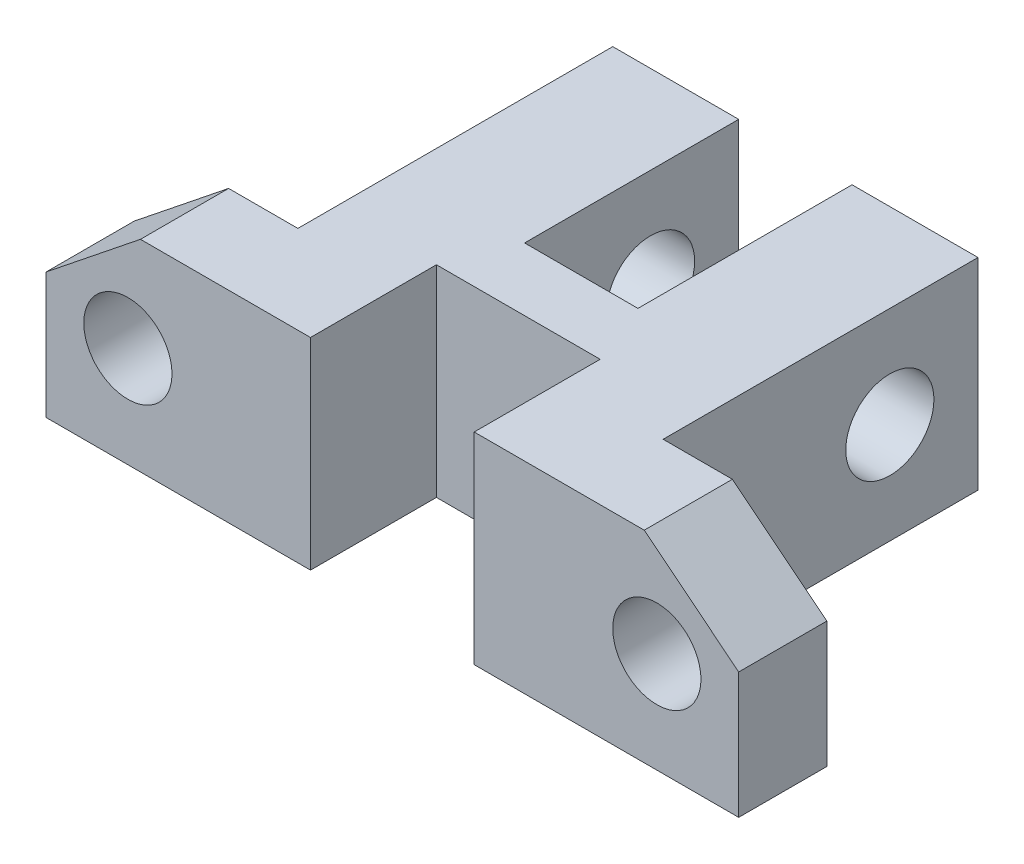
ISO-10303-21;
HEADER;
FILE_DESCRIPTION(('STEP AP214'),'2;1');
FILE_NAME('part.step','',(''),(''),'','','');
FILE_SCHEMA(('AUTOMOTIVE_DESIGN { 1 0 10303 214 1 1 1 1 }'));
ENDSEC;
DATA;
#1=APPLICATION_CONTEXT('core data for automotive mechanical design processes');
#2=APPLICATION_PROTOCOL_DEFINITION('international standard','automotive_design',2000,#1);
#3=PRODUCT_CONTEXT('',#1,'mechanical');
#4=PRODUCT('Part','Part','',(#3));
#5=PRODUCT_RELATED_PRODUCT_CATEGORY('part','',(#4));
#6=PRODUCT_DEFINITION_FORMATION('','',#4);
#7=PRODUCT_DEFINITION_CONTEXT('part definition',#1,'design');
#8=PRODUCT_DEFINITION('design','',#6,#7);
#9=PRODUCT_DEFINITION_SHAPE('','',#8);
#10=(LENGTH_UNIT() NAMED_UNIT(*) SI_UNIT(.MILLI.,.METRE.));
#11=(NAMED_UNIT(*) PLANE_ANGLE_UNIT() SI_UNIT($,.RADIAN.));
#12=(NAMED_UNIT(*) SI_UNIT($,.STERADIAN.) SOLID_ANGLE_UNIT());
#13=UNCERTAINTY_MEASURE_WITH_UNIT(LENGTH_MEASURE(1.E-05),#10,'distance_accuracy_value','');
#14=(GEOMETRIC_REPRESENTATION_CONTEXT(3) GLOBAL_UNCERTAINTY_ASSIGNED_CONTEXT((#13)) GLOBAL_UNIT_ASSIGNED_CONTEXT((#10,
#11,#12)) REPRESENTATION_CONTEXT('',''));
#15=CARTESIAN_POINT('',(0.,0.,0.));
#16=DIRECTION('',(0.,0.,1.));
#17=DIRECTION('',(1.,0.,0.));
#18=AXIS2_PLACEMENT_3D('',#15,#16,#17);
#19=CARTESIAN_POINT('',(0.,0.,32.));
#20=DIRECTION('',(0.,0.,-1.));
#21=DIRECTION('',(-1.,0.,0.));
#22=AXIS2_PLACEMENT_3D('',#19,#20,#21);
#23=PLANE('',#22);
#24=CARTESIAN_POINT('',(-21.,0.,32.));
#25=DIRECTION('',(0.,0.,-1.));
#26=DIRECTION('',(-1.,0.,0.));
#27=AXIS2_PLACEMENT_3D('',#24,#25,#26);
#28=CIRCLE('',#27,3.5);
#29=CARTESIAN_POINT('',(-24.5,0.,32.));
#30=VERTEX_POINT('',#29);
#31=EDGE_CURVE('E267',#30,#30,#28,.T.);
#32=ORIENTED_EDGE('',*,*,#31,.T.);
#33=EDGE_LOOP('',(#32));
#34=FACE_BOUND('',#33,.T.);
#35=DIRECTION('',(0.78086880944303,0.624695047554424,0.));
#36=VECTOR('',#35,1.);
#37=CARTESIAN_POINT('',(-11.7073170731707,14.6341463414634,32.));
#38=LINE('',#37,#36);
#39=CARTESIAN_POINT('',(-27.5,2.,32.));
#40=VERTEX_POINT('',#39);
#41=CARTESIAN_POINT('',(-20.,8.,32.));
#42=VERTEX_POINT('',#41);
#43=EDGE_CURVE('E266',#40,#42,#38,.T.);
#44=ORIENTED_EDGE('',*,*,#43,.F.);
#45=DIRECTION('',(0.,-1.,0.));
#46=VECTOR('',#45,1.);
#47=CARTESIAN_POINT('',(-27.5,8.,32.));
#48=LINE('',#47,#46);
#49=CARTESIAN_POINT('',(-27.5,-8.,32.));
#50=VERTEX_POINT('',#49);
#51=EDGE_CURVE('E192',#40,#50,#48,.T.);
#52=ORIENTED_EDGE('',*,*,#51,.T.);
#53=DIRECTION('',(1.,0.,0.));
#54=VECTOR('',#53,1.);
#55=CARTESIAN_POINT('',(-27.5,-8.,32.));
#56=LINE('',#55,#54);
#57=CARTESIAN_POINT('',(-6.5,-8.,32.));
#58=VERTEX_POINT('',#57);
#59=EDGE_CURVE('E190',#50,#58,#56,.T.);
#60=ORIENTED_EDGE('',*,*,#59,.T.);
#61=DIRECTION('',(0.,1.,0.));
#62=VECTOR('',#61,1.);
#63=CARTESIAN_POINT('',(-6.5,-8.,32.));
#64=LINE('',#63,#62);
#65=CARTESIAN_POINT('',(-6.5,8.,32.));
#66=VERTEX_POINT('',#65);
#67=EDGE_CURVE('E301',#58,#66,#64,.T.);
#68=ORIENTED_EDGE('',*,*,#67,.T.);
#69=DIRECTION('',(1.,0.,0.));
#70=VECTOR('',#69,1.);
#71=CARTESIAN_POINT('',(-27.5,8.,32.));
#72=LINE('',#71,#70);
#73=EDGE_CURVE('E187',#42,#66,#72,.T.);
#74=ORIENTED_EDGE('',*,*,#73,.F.);
#75=EDGE_LOOP('',(#44,#52,#60,#68,#74));
#76=FACE_BOUND('',#75,.T.);
#77=ADVANCED_FACE('F39',(#34,#76),#23,.F.);
#78=CARTESIAN_POINT('',(27.5,8.,32.));
#79=DIRECTION('',(1.,0.,0.));
#80=DIRECTION('',(0.,1.,0.));
#81=AXIS2_PLACEMENT_3D('',#78,#79,#80);
#82=PLANE('',#81);
#83=DIRECTION('',(0.,1.,0.));
#84=VECTOR('',#83,1.);
#85=CARTESIAN_POINT('',(27.5,-8.,25.));
#86=LINE('',#85,#84);
#87=CARTESIAN_POINT('',(27.5,-8.,25.));
#88=VERTEX_POINT('',#87);
#89=CARTESIAN_POINT('',(27.5,2.,25.));
#90=VERTEX_POINT('',#89);
#91=EDGE_CURVE('E178',#88,#90,#86,.T.);
#92=ORIENTED_EDGE('',*,*,#91,.T.);
#93=DIRECTION('',(0.,0.,-1.));
#94=VECTOR('',#93,1.);
#95=CARTESIAN_POINT('',(27.5,2.,32.));
#96=LINE('',#95,#94);
#97=CARTESIAN_POINT('',(27.5,2.,32.));
#98=VERTEX_POINT('',#97);
#99=EDGE_CURVE('E54',#98,#90,#96,.T.);
#100=ORIENTED_EDGE('',*,*,#99,.F.);
#101=DIRECTION('',(0.,-1.,0.));
#102=VECTOR('',#101,1.);
#103=CARTESIAN_POINT('',(27.5,8.,32.));
#104=LINE('',#103,#102);
#105=CARTESIAN_POINT('',(27.5,-8.,32.));
#106=VERTEX_POINT('',#105);
#107=EDGE_CURVE('E176',#98,#106,#104,.T.);
#108=ORIENTED_EDGE('',*,*,#107,.T.);
#109=DIRECTION('',(0.,0.,-1.));
#110=VECTOR('',#109,1.);
#111=CARTESIAN_POINT('',(27.5,-8.,32.));
#112=LINE('',#111,#110);
#113=EDGE_CURVE('E48',#106,#88,#112,.T.);
#114=ORIENTED_EDGE('',*,*,#113,.T.);
#115=EDGE_LOOP('',(#92,#100,#108,#114));
#116=FACE_BOUND('',#115,.T.);
#117=ADVANCED_FACE('F174',(#116),#82,.T.);
#118=CARTESIAN_POINT('',(-27.5,8.,32.));
#119=DIRECTION('',(0.,1.,0.));
#120=DIRECTION('',(0.,0.,1.));
#121=AXIS2_PLACEMENT_3D('',#118,#119,#120);
#122=PLANE('',#121);
#123=CARTESIAN_POINT('',(6.5,8.,32.));
#124=VERTEX_POINT('',#123);
#125=CARTESIAN_POINT('',(20.,8.,32.));
#126=VERTEX_POINT('',#125);
#127=EDGE_CURVE('E188',#124,#126,#72,.T.);
#128=ORIENTED_EDGE('',*,*,#127,.T.);
#129=DIRECTION('',(0.,0.,-1.));
#130=VECTOR('',#129,1.);
#131=CARTESIAN_POINT('',(20.,8.,32.));
#132=LINE('',#131,#130);
#133=CARTESIAN_POINT('',(20.,8.,25.));
#134=VERTEX_POINT('',#133);
#135=EDGE_CURVE('E167',#126,#134,#132,.T.);
#136=ORIENTED_EDGE('',*,*,#135,.T.);
#137=DIRECTION('',(1.,0.,0.));
#138=VECTOR('',#137,1.);
#139=CARTESIAN_POINT('',(-27.5,8.,25.));
#140=LINE('',#139,#138);
#141=CARTESIAN_POINT('',(14.5,8.,25.));
#142=VERTEX_POINT('',#141);
#143=EDGE_CURVE('E11',#142,#134,#140,.T.);
#144=ORIENTED_EDGE('',*,*,#143,.F.);
#145=DIRECTION('',(0.,0.,1.));
#146=VECTOR('',#145,1.);
#147=CARTESIAN_POINT('',(14.5,8.,32.));
#148=LINE('',#147,#146);
#149=CARTESIAN_POINT('',(14.5,8.,0.));
#150=VERTEX_POINT('',#149);
#151=EDGE_CURVE('E229',#150,#142,#148,.T.);
#152=ORIENTED_EDGE('',*,*,#151,.F.);
#153=DIRECTION('',(1.,0.,0.));
#154=VECTOR('',#153,1.);
#155=CARTESIAN_POINT('',(-27.5,8.,0.));
#156=LINE('',#155,#154);
#157=CARTESIAN_POINT('',(4.5,8.,0.));
#158=VERTEX_POINT('',#157);
#159=EDGE_CURVE('E203',#158,#150,#156,.T.);
#160=ORIENTED_EDGE('',*,*,#159,.F.);
#161=DIRECTION('',(0.,0.,-1.));
#162=VECTOR('',#161,1.);
#163=CARTESIAN_POINT('',(4.5,8.,0.));
#164=LINE('',#163,#162);
#165=CARTESIAN_POINT('',(4.5,8.,17.));
#166=VERTEX_POINT('',#165);
#167=EDGE_CURVE('E258',#166,#158,#164,.T.);
#168=ORIENTED_EDGE('',*,*,#167,.F.);
#169=DIRECTION('',(1.,0.,0.));
#170=VECTOR('',#169,1.);
#171=CARTESIAN_POINT('',(-4.5,8.,17.));
#172=LINE('',#171,#170);
#173=CARTESIAN_POINT('',(-4.5,8.,17.));
#174=VERTEX_POINT('',#173);
#175=EDGE_CURVE('E285',#174,#166,#172,.T.);
#176=ORIENTED_EDGE('',*,*,#175,.F.);
#177=DIRECTION('',(0.,0.,1.));
#178=VECTOR('',#177,1.);
#179=CARTESIAN_POINT('',(-4.5,8.,0.));
#180=LINE('',#179,#178);
#181=CARTESIAN_POINT('',(-4.5,8.,0.));
#182=VERTEX_POINT('',#181);
#183=EDGE_CURVE('E262',#182,#174,#180,.T.);
#184=ORIENTED_EDGE('',*,*,#183,.F.);
#185=CARTESIAN_POINT('',(-14.5,8.,0.));
#186=VERTEX_POINT('',#185);
#187=EDGE_CURVE('E201',#186,#182,#156,.T.);
#188=ORIENTED_EDGE('',*,*,#187,.F.);
#189=DIRECTION('',(0.,0.,-1.));
#190=VECTOR('',#189,1.);
#191=CARTESIAN_POINT('',(-14.5,8.,32.));
#192=LINE('',#191,#190);
#193=CARTESIAN_POINT('',(-14.5,8.,25.));
#194=VERTEX_POINT('',#193);
#195=EDGE_CURVE('E231',#194,#186,#192,.T.);
#196=ORIENTED_EDGE('',*,*,#195,.F.);
#197=DIRECTION('',(1.,0.,0.));
#198=VECTOR('',#197,1.);
#199=CARTESIAN_POINT('',(-27.5,8.,25.));
#200=LINE('',#199,#198);
#201=CARTESIAN_POINT('',(-20.,8.,25.));
#202=VERTEX_POINT('',#201);
#203=EDGE_CURVE('E233',#202,#194,#200,.T.);
#204=ORIENTED_EDGE('',*,*,#203,.F.);
#205=DIRECTION('',(0.,0.,-1.));
#206=VECTOR('',#205,1.);
#207=CARTESIAN_POINT('',(-20.,8.,32.));
#208=LINE('',#207,#206);
#209=EDGE_CURVE('E61',#42,#202,#208,.T.);
#210=ORIENTED_EDGE('',*,*,#209,.F.);
#211=ORIENTED_EDGE('',*,*,#73,.T.);
#212=DIRECTION('',(0.,0.,1.));
#213=VECTOR('',#212,1.);
#214=CARTESIAN_POINT('',(-6.5,8.,32.));
#215=LINE('',#214,#213);
#216=CARTESIAN_POINT('',(-6.5,8.,22.));
#217=VERTEX_POINT('',#216);
#218=EDGE_CURVE('E290',#217,#66,#215,.T.);
#219=ORIENTED_EDGE('',*,*,#218,.F.);
#220=DIRECTION('',(-1.,0.,0.));
#221=VECTOR('',#220,1.);
#222=CARTESIAN_POINT('',(-6.5,8.,22.));
#223=LINE('',#222,#221);
#224=CARTESIAN_POINT('',(6.5,8.,22.));
#225=VERTEX_POINT('',#224);
#226=EDGE_CURVE('E300',#225,#217,#223,.T.);
#227=ORIENTED_EDGE('',*,*,#226,.F.);
#228=DIRECTION('',(0.,0.,-1.));
#229=VECTOR('',#228,1.);
#230=CARTESIAN_POINT('',(6.5,8.,32.));
#231=LINE('',#230,#229);
#232=EDGE_CURVE('E302',#124,#225,#231,.T.);
#233=ORIENTED_EDGE('',*,*,#232,.F.);
#234=EDGE_LOOP('',(#128,#136,#144,#152,#160,#168,#176,#184,#188,#196,#204,#210,#211,#219,#227,#233));
#235=FACE_BOUND('',#234,.T.);
#236=ADVANCED_FACE('F255',(#235),#122,.T.);
#237=CARTESIAN_POINT('',(-27.5,8.,32.));
#238=DIRECTION('',(1.,0.,0.));
#239=DIRECTION('',(0.,1.,0.));
#240=AXIS2_PLACEMENT_3D('',#237,#238,#239);
#241=PLANE('',#240);
#242=DIRECTION('',(0.,0.,-1.));
#243=VECTOR('',#242,1.);
#244=CARTESIAN_POINT('',(-27.5,2.,32.));
#245=LINE('',#244,#243);
#246=CARTESIAN_POINT('',(-27.5,2.,25.));
#247=VERTEX_POINT('',#246);
#248=EDGE_CURVE('E257',#40,#247,#245,.T.);
#249=ORIENTED_EDGE('',*,*,#248,.T.);
#250=DIRECTION('',(0.,1.,0.));
#251=VECTOR('',#250,1.);
#252=CARTESIAN_POINT('',(-27.5,-8.,25.));
#253=LINE('',#252,#251);
#254=CARTESIAN_POINT('',(-27.5,-8.,25.));
#255=VERTEX_POINT('',#254);
#256=EDGE_CURVE('E325',#255,#247,#253,.T.);
#257=ORIENTED_EDGE('',*,*,#256,.F.);
#258=DIRECTION('',(0.,0.,-1.));
#259=VECTOR('',#258,1.);
#260=CARTESIAN_POINT('',(-27.5,-8.,32.));
#261=LINE('',#260,#259);
#262=EDGE_CURVE('E197',#50,#255,#261,.T.);
#263=ORIENTED_EDGE('',*,*,#262,.F.);
#264=ORIENTED_EDGE('',*,*,#51,.F.);
#265=EDGE_LOOP('',(#249,#257,#263,#264));
#266=FACE_BOUND('',#265,.T.);
#267=ADVANCED_FACE('F332',(#266),#241,.F.);
#268=CARTESIAN_POINT('',(21.,0.,32.));
#269=DIRECTION('',(0.,0.,-1.));
#270=DIRECTION('',(-1.,0.,0.));
#271=AXIS2_PLACEMENT_3D('',#268,#269,#270);
#272=CIRCLE('',#271,3.5);
#273=CARTESIAN_POINT('',(17.5,0.,32.));
#274=VERTEX_POINT('',#273);
#275=EDGE_CURVE('E395',#274,#274,#272,.F.);
#276=ORIENTED_EDGE('',*,*,#275,.F.);
#277=EDGE_LOOP('',(#276));
#278=FACE_BOUND('',#277,.T.);
#279=DIRECTION('',(0.78086880944303,-0.624695047554425,0.));
#280=VECTOR('',#279,1.);
#281=CARTESIAN_POINT('',(11.7073170731707,14.6341463414634,32.));
#282=LINE('',#281,#280);
#283=EDGE_CURVE('E162',#126,#98,#282,.T.);
#284=ORIENTED_EDGE('',*,*,#283,.F.);
#285=ORIENTED_EDGE('',*,*,#127,.F.);
#286=DIRECTION('',(0.,1.,0.));
#287=VECTOR('',#286,1.);
#288=CARTESIAN_POINT('',(6.5,-8.,32.));
#289=LINE('',#288,#287);
#290=CARTESIAN_POINT('',(6.5,-8.,32.));
#291=VERTEX_POINT('',#290);
#292=EDGE_CURVE('E311',#291,#124,#289,.T.);
#293=ORIENTED_EDGE('',*,*,#292,.F.);
#294=EDGE_CURVE('E184',#291,#106,#56,.T.);
#295=ORIENTED_EDGE('',*,*,#294,.T.);
#296=ORIENTED_EDGE('',*,*,#107,.F.);
#297=EDGE_LOOP('',(#284,#285,#293,#295,#296));
#298=FACE_BOUND('',#297,.T.);
#299=ADVANCED_FACE('F182',(#278,#298),#23,.F.);
#300=CARTESIAN_POINT('',(27.5,-8.,25.));
#301=DIRECTION('',(0.,0.,1.));
#302=DIRECTION('',(1.,0.,0.));
#303=AXIS2_PLACEMENT_3D('',#300,#301,#302);
#304=PLANE('',#303);
#305=CARTESIAN_POINT('',(21.,0.,25.));
#306=DIRECTION('',(0.,0.,-1.));
#307=DIRECTION('',(-1.,0.,0.));
#308=AXIS2_PLACEMENT_3D('',#305,#306,#307);
#309=CIRCLE('',#308,3.5);
#310=CARTESIAN_POINT('',(17.5,0.,25.));
#311=VERTEX_POINT('',#310);
#312=EDGE_CURVE('E394',#311,#311,#309,.F.);
#313=ORIENTED_EDGE('',*,*,#312,.T.);
#314=EDGE_LOOP('',(#313));
#315=FACE_BOUND('',#314,.T.);
#316=DIRECTION('',(0.78086880944303,-0.624695047554425,0.));
#317=VECTOR('',#316,1.);
#318=CARTESIAN_POINT('',(11.7073170731707,14.6341463414634,25.));
#319=LINE('',#318,#317);
#320=EDGE_CURVE('E173',#134,#90,#319,.T.);
#321=ORIENTED_EDGE('',*,*,#320,.T.);
#322=ORIENTED_EDGE('',*,*,#91,.F.);
#323=DIRECTION('',(1.,0.,0.));
#324=VECTOR('',#323,1.);
#325=CARTESIAN_POINT('',(27.5,-8.,25.));
#326=LINE('',#325,#324);
#327=CARTESIAN_POINT('',(14.5,-8.,25.));
#328=VERTEX_POINT('',#327);
#329=EDGE_CURVE('E213',#328,#88,#326,.T.);
#330=ORIENTED_EDGE('',*,*,#329,.F.);
#331=DIRECTION('',(0.,1.,0.));
#332=VECTOR('',#331,1.);
#333=CARTESIAN_POINT('',(14.5,-8.,25.));
#334=LINE('',#333,#332);
#335=EDGE_CURVE('E222',#328,#142,#334,.T.);
#336=ORIENTED_EDGE('',*,*,#335,.T.);
#337=ORIENTED_EDGE('',*,*,#143,.T.);
#338=EDGE_LOOP('',(#321,#322,#330,#336,#337));
#339=FACE_BOUND('',#338,.T.);
#340=ADVANCED_FACE('F256',(#315,#339),#304,.F.);
#341=CARTESIAN_POINT('',(-27.5,-8.,25.));
#342=DIRECTION('',(0.,0.,1.));
#343=DIRECTION('',(1.,0.,0.));
#344=AXIS2_PLACEMENT_3D('',#341,#342,#343);
#345=PLANE('',#344);
#346=CARTESIAN_POINT('',(-21.,0.,25.));
#347=DIRECTION('',(0.,0.,-1.));
#348=DIRECTION('',(-1.,0.,0.));
#349=AXIS2_PLACEMENT_3D('',#346,#347,#348);
#350=CIRCLE('',#349,3.5);
#351=CARTESIAN_POINT('',(-24.5,0.,25.));
#352=VERTEX_POINT('',#351);
#353=EDGE_CURVE('E392',#352,#352,#350,.T.);
#354=ORIENTED_EDGE('',*,*,#353,.F.);
#355=EDGE_LOOP('',(#354));
#356=FACE_BOUND('',#355,.T.);
#357=DIRECTION('',(0.78086880944303,0.624695047554424,0.));
#358=VECTOR('',#357,1.);
#359=CARTESIAN_POINT('',(-11.7073170731707,14.6341463414634,25.));
#360=LINE('',#359,#358);
#361=EDGE_CURVE('E268',#247,#202,#360,.T.);
#362=ORIENTED_EDGE('',*,*,#361,.T.);
#363=ORIENTED_EDGE('',*,*,#203,.T.);
#364=DIRECTION('',(0.,1.,0.));
#365=VECTOR('',#364,1.);
#366=CARTESIAN_POINT('',(-14.5,-8.,25.));
#367=LINE('',#366,#365);
#368=CARTESIAN_POINT('',(-14.5,-8.,25.));
#369=VERTEX_POINT('',#368);
#370=EDGE_CURVE('E324',#369,#194,#367,.T.);
#371=ORIENTED_EDGE('',*,*,#370,.F.);
#372=DIRECTION('',(1.,0.,0.));
#373=VECTOR('',#372,1.);
#374=CARTESIAN_POINT('',(-27.5,-8.,25.));
#375=LINE('',#374,#373);
#376=EDGE_CURVE('E226',#255,#369,#375,.T.);
#377=ORIENTED_EDGE('',*,*,#376,.F.);
#378=ORIENTED_EDGE('',*,*,#256,.T.);
#379=EDGE_LOOP('',(#362,#363,#371,#377,#378));
#380=FACE_BOUND('',#379,.T.);
#381=ADVANCED_FACE('F327',(#356,#380),#345,.F.);
#382=CARTESIAN_POINT('',(0.,0.,0.));
#383=DIRECTION('',(0.,0.,-1.));
#384=DIRECTION('',(-1.,0.,0.));
#385=AXIS2_PLACEMENT_3D('',#382,#383,#384);
#386=PLANE('',#385);
#387=DIRECTION('',(0.,1.,0.));
#388=VECTOR('',#387,1.);
#389=CARTESIAN_POINT('',(-4.5,-8.,0.));
#390=LINE('',#389,#388);
#391=CARTESIAN_POINT('',(-4.5,-8.,0.));
#392=VERTEX_POINT('',#391);
#393=EDGE_CURVE('E289',#392,#182,#390,.T.);
#394=ORIENTED_EDGE('',*,*,#393,.F.);
#395=DIRECTION('',(1.,0.,0.));
#396=VECTOR('',#395,1.);
#397=CARTESIAN_POINT('',(-27.5,-8.,0.));
#398=LINE('',#397,#396);
#399=CARTESIAN_POINT('',(-14.5,-8.,0.));
#400=VERTEX_POINT('',#399);
#401=EDGE_CURVE('E196',#400,#392,#398,.T.);
#402=ORIENTED_EDGE('',*,*,#401,.F.);
#403=DIRECTION('',(0.,1.,0.));
#404=VECTOR('',#403,1.);
#405=CARTESIAN_POINT('',(-14.5,-8.,0.));
#406=LINE('',#405,#404);
#407=EDGE_CURVE('E235',#400,#186,#406,.T.);
#408=ORIENTED_EDGE('',*,*,#407,.T.);
#409=ORIENTED_EDGE('',*,*,#187,.T.);
#410=EDGE_LOOP('',(#394,#402,#408,#409));
#411=FACE_BOUND('',#410,.T.);
#412=ADVANCED_FACE('F349',(#411),#386,.T.);
#413=CARTESIAN_POINT('',(-27.5,-8.,32.));
#414=DIRECTION('',(0.,1.,0.));
#415=DIRECTION('',(0.,0.,1.));
#416=AXIS2_PLACEMENT_3D('',#413,#414,#415);
#417=PLANE('',#416);
#418=ORIENTED_EDGE('',*,*,#401,.T.);
#419=DIRECTION('',(0.,0.,1.));
#420=VECTOR('',#419,1.);
#421=CARTESIAN_POINT('',(-4.5,-8.,0.));
#422=LINE('',#421,#420);
#423=CARTESIAN_POINT('',(-4.5,-8.,17.));
#424=VERTEX_POINT('',#423);
#425=EDGE_CURVE('E272',#392,#424,#422,.T.);
#426=ORIENTED_EDGE('',*,*,#425,.T.);
#427=DIRECTION('',(1.,0.,0.));
#428=VECTOR('',#427,1.);
#429=CARTESIAN_POINT('',(-4.5,-8.,17.));
#430=LINE('',#429,#428);
#431=CARTESIAN_POINT('',(4.5,-8.,17.));
#432=VERTEX_POINT('',#431);
#433=EDGE_CURVE('E277',#424,#432,#430,.T.);
#434=ORIENTED_EDGE('',*,*,#433,.T.);
#435=DIRECTION('',(0.,0.,-1.));
#436=VECTOR('',#435,1.);
#437=CARTESIAN_POINT('',(4.5,-8.,0.));
#438=LINE('',#437,#436);
#439=CARTESIAN_POINT('',(4.5,-8.,0.));
#440=VERTEX_POINT('',#439);
#441=EDGE_CURVE('E245',#432,#440,#438,.T.);
#442=ORIENTED_EDGE('',*,*,#441,.T.);
#443=CARTESIAN_POINT('',(14.5,-8.,0.));
#444=VERTEX_POINT('',#443);
#445=EDGE_CURVE('E205',#440,#444,#398,.T.);
#446=ORIENTED_EDGE('',*,*,#445,.T.);
#447=DIRECTION('',(0.,0.,1.));
#448=VECTOR('',#447,1.);
#449=CARTESIAN_POINT('',(14.5,-8.,0.));
#450=LINE('',#449,#448);
#451=EDGE_CURVE('E214',#444,#328,#450,.T.);
#452=ORIENTED_EDGE('',*,*,#451,.T.);
#453=ORIENTED_EDGE('',*,*,#329,.T.);
#454=ORIENTED_EDGE('',*,*,#113,.F.);
#455=ORIENTED_EDGE('',*,*,#294,.F.);
#456=DIRECTION('',(0.,0.,-1.));
#457=VECTOR('',#456,1.);
#458=CARTESIAN_POINT('',(6.5,-8.,32.));
#459=LINE('',#458,#457);
#460=CARTESIAN_POINT('',(6.5,-8.,22.));
#461=VERTEX_POINT('',#460);
#462=EDGE_CURVE('E298',#291,#461,#459,.T.);
#463=ORIENTED_EDGE('',*,*,#462,.T.);
#464=DIRECTION('',(-1.,0.,0.));
#465=VECTOR('',#464,1.);
#466=CARTESIAN_POINT('',(-6.5,-8.,22.));
#467=LINE('',#466,#465);
#468=CARTESIAN_POINT('',(-6.5,-8.,22.));
#469=VERTEX_POINT('',#468);
#470=EDGE_CURVE('E297',#461,#469,#467,.T.);
#471=ORIENTED_EDGE('',*,*,#470,.T.);
#472=DIRECTION('',(0.,0.,1.));
#473=VECTOR('',#472,1.);
#474=CARTESIAN_POINT('',(-6.5,-8.,32.));
#475=LINE('',#474,#473);
#476=EDGE_CURVE('E291',#469,#58,#475,.T.);
#477=ORIENTED_EDGE('',*,*,#476,.T.);
#478=ORIENTED_EDGE('',*,*,#59,.F.);
#479=ORIENTED_EDGE('',*,*,#262,.T.);
#480=ORIENTED_EDGE('',*,*,#376,.T.);
#481=DIRECTION('',(0.,0.,-1.));
#482=VECTOR('',#481,1.);
#483=CARTESIAN_POINT('',(-14.5,-8.,0.));
#484=LINE('',#483,#482);
#485=EDGE_CURVE('E317',#369,#400,#484,.T.);
#486=ORIENTED_EDGE('',*,*,#485,.T.);
#487=EDGE_LOOP('',(#418,#426,#434,#442,#446,#452,#453,#454,#455,#463,#471,#477,#478,#479,#480,#486));
#488=FACE_BOUND('',#487,.T.);
#489=ADVANCED_FACE('F41',(#488),#417,.F.);
#490=DIRECTION('',(0.,1.,0.));
#491=VECTOR('',#490,1.);
#492=CARTESIAN_POINT('',(4.5,-8.,0.));
#493=LINE('',#492,#491);
#494=EDGE_CURVE('E253',#440,#158,#493,.T.);
#495=ORIENTED_EDGE('',*,*,#494,.T.);
#496=ORIENTED_EDGE('',*,*,#159,.T.);
#497=DIRECTION('',(0.,1.,0.));
#498=VECTOR('',#497,1.);
#499=CARTESIAN_POINT('',(14.5,-8.,0.));
#500=LINE('',#499,#498);
#501=EDGE_CURVE('E217',#444,#150,#500,.T.);
#502=ORIENTED_EDGE('',*,*,#501,.F.);
#503=ORIENTED_EDGE('',*,*,#445,.F.);
#504=EDGE_LOOP('',(#495,#496,#502,#503));
#505=FACE_BOUND('',#504,.T.);
#506=ADVANCED_FACE('F248',(#505),#386,.T.);
#507=CARTESIAN_POINT('',(14.5,-8.,0.));
#508=DIRECTION('',(-1.,0.,0.));
#509=DIRECTION('',(0.,0.,1.));
#510=AXIS2_PLACEMENT_3D('',#507,#508,#509);
#511=PLANE('',#510);
#512=CARTESIAN_POINT('',(14.5,0.,7.));
#513=DIRECTION('',(1.,0.,0.));
#514=DIRECTION('',(0.,0.,-1.));
#515=AXIS2_PLACEMENT_3D('',#512,#513,#514);
#516=CIRCLE('',#515,3.5);
#517=CARTESIAN_POINT('',(14.5,0.,3.5));
#518=VERTEX_POINT('',#517);
#519=EDGE_CURVE('E406',#518,#518,#516,.T.);
#520=ORIENTED_EDGE('',*,*,#519,.F.);
#521=EDGE_LOOP('',(#520));
#522=FACE_BOUND('',#521,.T.);
#523=ORIENTED_EDGE('',*,*,#151,.T.);
#524=ORIENTED_EDGE('',*,*,#335,.F.);
#525=ORIENTED_EDGE('',*,*,#451,.F.);
#526=ORIENTED_EDGE('',*,*,#501,.T.);
#527=EDGE_LOOP('',(#523,#524,#525,#526));
#528=FACE_BOUND('',#527,.T.);
#529=ADVANCED_FACE('F246',(#522,#528),#511,.F.);
#530=CARTESIAN_POINT('',(-14.5,-8.,0.));
#531=DIRECTION('',(1.,0.,0.));
#532=DIRECTION('',(0.,0.,-1.));
#533=AXIS2_PLACEMENT_3D('',#530,#531,#532);
#534=PLANE('',#533);
#535=CARTESIAN_POINT('',(-14.5,0.,7.));
#536=DIRECTION('',(1.,0.,0.));
#537=DIRECTION('',(0.,0.,-1.));
#538=AXIS2_PLACEMENT_3D('',#535,#536,#537);
#539=CIRCLE('',#538,3.5);
#540=CARTESIAN_POINT('',(-14.5,0.,3.5));
#541=VERTEX_POINT('',#540);
#542=EDGE_CURVE('E397',#541,#541,#539,.T.);
#543=ORIENTED_EDGE('',*,*,#542,.T.);
#544=EDGE_LOOP('',(#543));
#545=FACE_BOUND('',#544,.T.);
#546=ORIENTED_EDGE('',*,*,#195,.T.);
#547=ORIENTED_EDGE('',*,*,#407,.F.);
#548=ORIENTED_EDGE('',*,*,#485,.F.);
#549=ORIENTED_EDGE('',*,*,#370,.T.);
#550=EDGE_LOOP('',(#546,#547,#548,#549));
#551=FACE_BOUND('',#550,.T.);
#552=ADVANCED_FACE('F343',(#545,#551),#534,.F.);
#553=CARTESIAN_POINT('',(-6.5,-8.,32.));
#554=DIRECTION('',(-1.,0.,0.));
#555=DIRECTION('',(0.,0.,1.));
#556=AXIS2_PLACEMENT_3D('',#553,#554,#555);
#557=PLANE('',#556);
#558=ORIENTED_EDGE('',*,*,#218,.T.);
#559=ORIENTED_EDGE('',*,*,#67,.F.);
#560=ORIENTED_EDGE('',*,*,#476,.F.);
#561=DIRECTION('',(0.,1.,0.));
#562=VECTOR('',#561,1.);
#563=CARTESIAN_POINT('',(-6.5,-8.,22.));
#564=LINE('',#563,#562);
#565=EDGE_CURVE('E224',#469,#217,#564,.T.);
#566=ORIENTED_EDGE('',*,*,#565,.T.);
#567=EDGE_LOOP('',(#558,#559,#560,#566));
#568=FACE_BOUND('',#567,.T.);
#569=ADVANCED_FACE('F476',(#568),#557,.F.);
#570=CARTESIAN_POINT('',(-6.5,-8.,22.));
#571=DIRECTION('',(0.,0.,-1.));
#572=DIRECTION('',(-1.,0.,0.));
#573=AXIS2_PLACEMENT_3D('',#570,#571,#572);
#574=PLANE('',#573);
#575=ORIENTED_EDGE('',*,*,#226,.T.);
#576=ORIENTED_EDGE('',*,*,#565,.F.);
#577=ORIENTED_EDGE('',*,*,#470,.F.);
#578=DIRECTION('',(0.,1.,0.));
#579=VECTOR('',#578,1.);
#580=CARTESIAN_POINT('',(6.5,-8.,22.));
#581=LINE('',#580,#579);
#582=EDGE_CURVE('E313',#461,#225,#581,.T.);
#583=ORIENTED_EDGE('',*,*,#582,.T.);
#584=EDGE_LOOP('',(#575,#576,#577,#583));
#585=FACE_BOUND('',#584,.T.);
#586=ADVANCED_FACE('F568',(#585),#574,.F.);
#587=CARTESIAN_POINT('',(6.5,-8.,32.));
#588=DIRECTION('',(1.,0.,0.));
#589=DIRECTION('',(0.,0.,-1.));
#590=AXIS2_PLACEMENT_3D('',#587,#588,#589);
#591=PLANE('',#590);
#592=ORIENTED_EDGE('',*,*,#232,.T.);
#593=ORIENTED_EDGE('',*,*,#582,.F.);
#594=ORIENTED_EDGE('',*,*,#462,.F.);
#595=ORIENTED_EDGE('',*,*,#292,.T.);
#596=EDGE_LOOP('',(#592,#593,#594,#595));
#597=FACE_BOUND('',#596,.T.);
#598=ADVANCED_FACE('F368',(#597),#591,.F.);
#599=CARTESIAN_POINT('',(-4.5,-8.,0.));
#600=DIRECTION('',(-1.,0.,0.));
#601=DIRECTION('',(0.,0.,1.));
#602=AXIS2_PLACEMENT_3D('',#599,#600,#601);
#603=PLANE('',#602);
#604=CARTESIAN_POINT('',(-4.5,0.,7.));
#605=DIRECTION('',(-1.,0.,0.));
#606=DIRECTION('',(0.,0.,1.));
#607=AXIS2_PLACEMENT_3D('',#604,#605,#606);
#608=CIRCLE('',#607,3.5);
#609=CARTESIAN_POINT('',(-4.5,0.,10.5));
#610=VERTEX_POINT('',#609);
#611=EDGE_CURVE('E403',#610,#610,#608,.T.);
#612=ORIENTED_EDGE('',*,*,#611,.T.);
#613=EDGE_LOOP('',(#612));
#614=FACE_BOUND('',#613,.T.);
#615=ORIENTED_EDGE('',*,*,#183,.T.);
#616=DIRECTION('',(0.,1.,0.));
#617=VECTOR('',#616,1.);
#618=CARTESIAN_POINT('',(-4.5,-8.,17.));
#619=LINE('',#618,#617);
#620=EDGE_CURVE('E276',#424,#174,#619,.T.);
#621=ORIENTED_EDGE('',*,*,#620,.F.);
#622=ORIENTED_EDGE('',*,*,#425,.F.);
#623=ORIENTED_EDGE('',*,*,#393,.T.);
#624=EDGE_LOOP('',(#615,#621,#622,#623));
#625=FACE_BOUND('',#624,.T.);
#626=ADVANCED_FACE('F355',(#614,#625),#603,.F.);
#627=CARTESIAN_POINT('',(4.5,-8.,0.));
#628=DIRECTION('',(1.,0.,0.));
#629=DIRECTION('',(0.,0.,-1.));
#630=AXIS2_PLACEMENT_3D('',#627,#628,#629);
#631=PLANE('',#630);
#632=CARTESIAN_POINT('',(4.5,0.,7.));
#633=DIRECTION('',(1.,0.,0.));
#634=DIRECTION('',(0.,0.,-1.));
#635=AXIS2_PLACEMENT_3D('',#632,#633,#634);
#636=CIRCLE('',#635,3.5);
#637=CARTESIAN_POINT('',(4.5,0.,3.5));
#638=VERTEX_POINT('',#637);
#639=EDGE_CURVE('E43',#638,#638,#636,.T.);
#640=ORIENTED_EDGE('',*,*,#639,.T.);
#641=EDGE_LOOP('',(#640));
#642=FACE_BOUND('',#641,.T.);
#643=ORIENTED_EDGE('',*,*,#167,.T.);
#644=ORIENTED_EDGE('',*,*,#494,.F.);
#645=ORIENTED_EDGE('',*,*,#441,.F.);
#646=DIRECTION('',(0.,1.,0.));
#647=VECTOR('',#646,1.);
#648=CARTESIAN_POINT('',(4.5,-8.,17.));
#649=LINE('',#648,#647);
#650=EDGE_CURVE('E287',#432,#166,#649,.T.);
#651=ORIENTED_EDGE('',*,*,#650,.T.);
#652=EDGE_LOOP('',(#643,#644,#645,#651));
#653=FACE_BOUND('',#652,.T.);
#654=ADVANCED_FACE('F359',(#642,#653),#631,.F.);
#655=CARTESIAN_POINT('',(-4.5,-8.,17.));
#656=DIRECTION('',(0.,0.,1.));
#657=DIRECTION('',(1.,0.,0.));
#658=AXIS2_PLACEMENT_3D('',#655,#656,#657);
#659=PLANE('',#658);
#660=ORIENTED_EDGE('',*,*,#175,.T.);
#661=ORIENTED_EDGE('',*,*,#650,.F.);
#662=ORIENTED_EDGE('',*,*,#433,.F.);
#663=ORIENTED_EDGE('',*,*,#620,.T.);
#664=EDGE_LOOP('',(#660,#661,#662,#663));
#665=FACE_BOUND('',#664,.T.);
#666=ADVANCED_FACE('F352',(#665),#659,.F.);
#667=CARTESIAN_POINT('',(-11.7073170731707,14.6341463414634,32.));
#668=DIRECTION('',(-0.624695047554424,0.78086880944303,0.));
#669=DIRECTION('',(-0.78086880944303,-0.624695047554424,0.));
#670=AXIS2_PLACEMENT_3D('',#667,#668,#669);
#671=PLANE('',#670);
#672=ORIENTED_EDGE('',*,*,#361,.F.);
#673=ORIENTED_EDGE('',*,*,#248,.F.);
#674=ORIENTED_EDGE('',*,*,#43,.T.);
#675=ORIENTED_EDGE('',*,*,#209,.T.);
#676=EDGE_LOOP('',(#672,#673,#674,#675));
#677=FACE_BOUND('',#676,.T.);
#678=ADVANCED_FACE('F336',(#677),#671,.T.);
#679=CARTESIAN_POINT('',(11.7073170731707,14.6341463414634,32.));
#680=DIRECTION('',(0.624695047554425,0.78086880944303,0.));
#681=DIRECTION('',(-0.78086880944303,0.624695047554425,0.));
#682=AXIS2_PLACEMENT_3D('',#679,#680,#681);
#683=PLANE('',#682);
#684=ORIENTED_EDGE('',*,*,#320,.F.);
#685=ORIENTED_EDGE('',*,*,#135,.F.);
#686=ORIENTED_EDGE('',*,*,#283,.T.);
#687=ORIENTED_EDGE('',*,*,#99,.T.);
#688=EDGE_LOOP('',(#684,#685,#686,#687));
#689=FACE_BOUND('',#688,.T.);
#690=ADVANCED_FACE('F163',(#689),#683,.T.);
#691=CARTESIAN_POINT('',(-21.,0.,32.));
#692=DIRECTION('',(0.,0.,-1.));
#693=DIRECTION('',(-1.,0.,0.));
#694=AXIS2_PLACEMENT_3D('',#691,#692,#693);
#695=CYLINDRICAL_SURFACE('',#694,3.5);
#696=CARTESIAN_POINT('',(-24.5,0.,32.));
#697=CARTESIAN_POINT('',(-24.5,0.,31.9270833333333));
#698=CARTESIAN_POINT('',(-24.5,0.,31.8541666666667));
#699=CARTESIAN_POINT('',(-24.5,0.,31.7083333333333));
#700=CARTESIAN_POINT('',(-24.5,0.,31.6354166666667));
#701=CARTESIAN_POINT('',(-24.5,0.,31.4895833333333));
#702=CARTESIAN_POINT('',(-24.5,0.,31.4166666666667));
#703=CARTESIAN_POINT('',(-24.5,0.,31.2708333333333));
#704=CARTESIAN_POINT('',(-24.5,0.,31.1979166666667));
#705=CARTESIAN_POINT('',(-24.5,0.,31.0520833333333));
#706=CARTESIAN_POINT('',(-24.5,0.,30.9791666666667));
#707=CARTESIAN_POINT('',(-24.5,0.,30.8333333333333));
#708=CARTESIAN_POINT('',(-24.5,0.,30.7604166666667));
#709=CARTESIAN_POINT('',(-24.5,0.,30.6145833333333));
#710=CARTESIAN_POINT('',(-24.5,0.,30.5416666666667));
#711=CARTESIAN_POINT('',(-24.5,0.,30.3958333333333));
#712=CARTESIAN_POINT('',(-24.5,0.,30.3229166666667));
#713=CARTESIAN_POINT('',(-24.5,0.,30.1770833333333));
#714=CARTESIAN_POINT('',(-24.5,0.,30.1041666666667));
#715=CARTESIAN_POINT('',(-24.5,0.,29.9583333333333));
#716=CARTESIAN_POINT('',(-24.5,0.,29.8854166666667));
#717=CARTESIAN_POINT('',(-24.5,0.,29.7395833333333));
#718=CARTESIAN_POINT('',(-24.5,0.,29.6666666666667));
#719=CARTESIAN_POINT('',(-24.5,0.,29.5208333333333));
#720=CARTESIAN_POINT('',(-24.5,0.,29.4479166666667));
#721=CARTESIAN_POINT('',(-24.5,0.,29.3020833333333));
#722=CARTESIAN_POINT('',(-24.5,0.,29.2291666666667));
#723=CARTESIAN_POINT('',(-24.5,0.,29.0833333333333));
#724=CARTESIAN_POINT('',(-24.5,0.,29.0104166666667));
#725=CARTESIAN_POINT('',(-24.5,0.,28.8645833333333));
#726=CARTESIAN_POINT('',(-24.5,0.,28.7916666666667));
#727=CARTESIAN_POINT('',(-24.5,0.,28.6458333333333));
#728=CARTESIAN_POINT('',(-24.5,0.,28.5729166666667));
#729=CARTESIAN_POINT('',(-24.5,0.,28.4270833333333));
#730=CARTESIAN_POINT('',(-24.5,0.,28.3541666666667));
#731=CARTESIAN_POINT('',(-24.5,0.,28.2083333333333));
#732=CARTESIAN_POINT('',(-24.5,0.,28.1354166666667));
#733=CARTESIAN_POINT('',(-24.5,0.,27.9895833333333));
#734=CARTESIAN_POINT('',(-24.5,0.,27.9166666666667));
#735=CARTESIAN_POINT('',(-24.5,0.,27.7708333333333));
#736=CARTESIAN_POINT('',(-24.5,0.,27.6979166666667));
#737=CARTESIAN_POINT('',(-24.5,0.,27.5520833333333));
#738=CARTESIAN_POINT('',(-24.5,0.,27.4791666666667));
#739=CARTESIAN_POINT('',(-24.5,0.,27.3333333333333));
#740=CARTESIAN_POINT('',(-24.5,0.,27.2604166666667));
#741=CARTESIAN_POINT('',(-24.5,0.,27.1145833333333));
#742=CARTESIAN_POINT('',(-24.5,0.,27.0416666666667));
#743=CARTESIAN_POINT('',(-24.5,0.,26.8958333333333));
#744=CARTESIAN_POINT('',(-24.5,0.,26.8229166666667));
#745=CARTESIAN_POINT('',(-24.5,0.,26.6770833333333));
#746=CARTESIAN_POINT('',(-24.5,0.,26.6041666666667));
#747=CARTESIAN_POINT('',(-24.5,0.,26.4583333333333));
#748=CARTESIAN_POINT('',(-24.5,0.,26.3854166666667));
#749=CARTESIAN_POINT('',(-24.5,0.,26.2395833333333));
#750=CARTESIAN_POINT('',(-24.5,0.,26.1666666666667));
#751=CARTESIAN_POINT('',(-24.5,0.,26.0208333333333));
#752=CARTESIAN_POINT('',(-24.5,0.,25.9479166666667));
#753=CARTESIAN_POINT('',(-24.5,0.,25.8020833333333));
#754=CARTESIAN_POINT('',(-24.5,0.,25.7291666666667));
#755=CARTESIAN_POINT('',(-24.5,0.,25.5833333333333));
#756=CARTESIAN_POINT('',(-24.5,0.,25.5104166666667));
#757=CARTESIAN_POINT('',(-24.5,0.,25.3645833333333));
#758=CARTESIAN_POINT('',(-24.5,0.,25.2916666666667));
#759=CARTESIAN_POINT('',(-24.5,0.,25.1458333333333));
#760=CARTESIAN_POINT('',(-24.5,0.,25.0729166666667));
#761=CARTESIAN_POINT('',(-24.5,0.,25.));
#762=B_SPLINE_CURVE_WITH_KNOTS('',3,(#696,#697,#698,#699,#700,#701,#702,#703,#704,#705,#706,
#707,#708,#709,#710,#711,#712,#713,#714,#715,#716,#717,#718,#719,#720,#721,#722,#723,#724,#725,
#726,#727,#728,#729,#730,#731,#732,#733,#734,#735,#736,#737,#738,#739,#740,#741,#742,#743,#744,
#745,#746,#747,#748,#749,#750,#751,#752,#753,#754,#755,#756,#757,#758,#759,#760,#761),
.UNSPECIFIED.,.F.,.F.,(4,2,2,2,2,2,2,2,2,2,2,2,2,2,2,2,2,2,2,2,2,2,2,2,2,2,2,2,2,2,2,2,4),(0.,
0.218749999999997,0.437499999999993,0.656249999999997,0.874999999999997,1.09375,1.3125,1.53125,
1.75,1.96875,2.1875,2.40625,2.625,2.84375,3.0625,3.28125,3.5,3.71875,3.9375,4.15625,4.375,
4.59375,4.8125,5.03125,5.25,5.46874999999999,5.6875,5.90624999999999,6.125,6.34375,6.5625,
6.78125,7.),.UNSPECIFIED.);
#763=EDGE_CURVE('BSEAM421',#30,#352,#762,.T.);
#764=ORIENTED_EDGE('',*,*,#31,.F.);
#765=ORIENTED_EDGE('',*,*,#353,.T.);
#766=ORIENTED_EDGE('',*,*,#763,.T.);
#767=ORIENTED_EDGE('',*,*,#763,.F.);
#768=EDGE_LOOP('',(#764,#766,#765,#767));
#769=FACE_BOUND('',#768,.T.);
#770=ADVANCED_FACE('F421',(#769),#695,.F.);
#771=CARTESIAN_POINT('',(21.,0.,32.));
#772=DIRECTION('',(0.,0.,-1.));
#773=DIRECTION('',(-1.,0.,0.));
#774=AXIS2_PLACEMENT_3D('',#771,#772,#773);
#775=CYLINDRICAL_SURFACE('',#774,3.5);
#776=CARTESIAN_POINT('',(17.5,0.,32.));
#777=CARTESIAN_POINT('',(17.5,0.,31.9270833333333));
#778=CARTESIAN_POINT('',(17.5,0.,31.8541666666667));
#779=CARTESIAN_POINT('',(17.5,0.,31.7083333333333));
#780=CARTESIAN_POINT('',(17.5,0.,31.6354166666667));
#781=CARTESIAN_POINT('',(17.5,0.,31.4895833333333));
#782=CARTESIAN_POINT('',(17.5,0.,31.4166666666667));
#783=CARTESIAN_POINT('',(17.5,0.,31.2708333333333));
#784=CARTESIAN_POINT('',(17.5,0.,31.1979166666667));
#785=CARTESIAN_POINT('',(17.5,0.,31.0520833333333));
#786=CARTESIAN_POINT('',(17.5,0.,30.9791666666667));
#787=CARTESIAN_POINT('',(17.5,0.,30.8333333333333));
#788=CARTESIAN_POINT('',(17.5,0.,30.7604166666667));
#789=CARTESIAN_POINT('',(17.5,0.,30.6145833333333));
#790=CARTESIAN_POINT('',(17.5,0.,30.5416666666667));
#791=CARTESIAN_POINT('',(17.5,0.,30.3958333333333));
#792=CARTESIAN_POINT('',(17.5,0.,30.3229166666667));
#793=CARTESIAN_POINT('',(17.5,0.,30.1770833333333));
#794=CARTESIAN_POINT('',(17.5,0.,30.1041666666667));
#795=CARTESIAN_POINT('',(17.5,0.,29.9583333333333));
#796=CARTESIAN_POINT('',(17.5,0.,29.8854166666667));
#797=CARTESIAN_POINT('',(17.5,0.,29.7395833333333));
#798=CARTESIAN_POINT('',(17.5,0.,29.6666666666667));
#799=CARTESIAN_POINT('',(17.5,0.,29.5208333333333));
#800=CARTESIAN_POINT('',(17.5,0.,29.4479166666667));
#801=CARTESIAN_POINT('',(17.5,0.,29.3020833333333));
#802=CARTESIAN_POINT('',(17.5,0.,29.2291666666667));
#803=CARTESIAN_POINT('',(17.5,0.,29.0833333333333));
#804=CARTESIAN_POINT('',(17.5,0.,29.0104166666667));
#805=CARTESIAN_POINT('',(17.5,0.,28.8645833333333));
#806=CARTESIAN_POINT('',(17.5,0.,28.7916666666667));
#807=CARTESIAN_POINT('',(17.5,0.,28.6458333333333));
#808=CARTESIAN_POINT('',(17.5,0.,28.5729166666667));
#809=CARTESIAN_POINT('',(17.5,0.,28.4270833333333));
#810=CARTESIAN_POINT('',(17.5,0.,28.3541666666667));
#811=CARTESIAN_POINT('',(17.5,0.,28.2083333333333));
#812=CARTESIAN_POINT('',(17.5,0.,28.1354166666667));
#813=CARTESIAN_POINT('',(17.5,0.,27.9895833333333));
#814=CARTESIAN_POINT('',(17.5,0.,27.9166666666667));
#815=CARTESIAN_POINT('',(17.5,0.,27.7708333333333));
#816=CARTESIAN_POINT('',(17.5,0.,27.6979166666667));
#817=CARTESIAN_POINT('',(17.5,0.,27.5520833333333));
#818=CARTESIAN_POINT('',(17.5,0.,27.4791666666667));
#819=CARTESIAN_POINT('',(17.5,0.,27.3333333333333));
#820=CARTESIAN_POINT('',(17.5,0.,27.2604166666667));
#821=CARTESIAN_POINT('',(17.5,0.,27.1145833333333));
#822=CARTESIAN_POINT('',(17.5,0.,27.0416666666667));
#823=CARTESIAN_POINT('',(17.5,0.,26.8958333333333));
#824=CARTESIAN_POINT('',(17.5,0.,26.8229166666667));
#825=CARTESIAN_POINT('',(17.5,0.,26.6770833333333));
#826=CARTESIAN_POINT('',(17.5,0.,26.6041666666667));
#827=CARTESIAN_POINT('',(17.5,0.,26.4583333333333));
#828=CARTESIAN_POINT('',(17.5,0.,26.3854166666667));
#829=CARTESIAN_POINT('',(17.5,0.,26.2395833333333));
#830=CARTESIAN_POINT('',(17.5,0.,26.1666666666667));
#831=CARTESIAN_POINT('',(17.5,0.,26.0208333333333));
#832=CARTESIAN_POINT('',(17.5,0.,25.9479166666667));
#833=CARTESIAN_POINT('',(17.5,0.,25.8020833333333));
#834=CARTESIAN_POINT('',(17.5,0.,25.7291666666667));
#835=CARTESIAN_POINT('',(17.5,0.,25.5833333333333));
#836=CARTESIAN_POINT('',(17.5,0.,25.5104166666667));
#837=CARTESIAN_POINT('',(17.5,0.,25.3645833333333));
#838=CARTESIAN_POINT('',(17.5,0.,25.2916666666667));
#839=CARTESIAN_POINT('',(17.5,0.,25.1458333333333));
#840=CARTESIAN_POINT('',(17.5,0.,25.0729166666667));
#841=CARTESIAN_POINT('',(17.5,0.,25.));
#842=B_SPLINE_CURVE_WITH_KNOTS('',3,(#776,#777,#778,#779,#780,#781,#782,#783,#784,#785,#786,
#787,#788,#789,#790,#791,#792,#793,#794,#795,#796,#797,#798,#799,#800,#801,#802,#803,#804,#805,
#806,#807,#808,#809,#810,#811,#812,#813,#814,#815,#816,#817,#818,#819,#820,#821,#822,#823,#824,
#825,#826,#827,#828,#829,#830,#831,#832,#833,#834,#835,#836,#837,#838,#839,#840,#841),
.UNSPECIFIED.,.F.,.F.,(4,2,2,2,2,2,2,2,2,2,2,2,2,2,2,2,2,2,2,2,2,2,2,2,2,2,2,2,2,2,2,2,4),(0.,
0.218749999999997,0.437499999999993,0.656249999999997,0.874999999999997,1.09375,1.3125,1.53125,
1.75,1.96875,2.1875,2.40625,2.625,2.84375,3.0625,3.28125,3.5,3.71875,3.9375,4.15625,4.375,
4.59375,4.8125,5.03125,5.25,5.46874999999999,5.6875,5.90624999999999,6.125,6.34375,6.5625,
6.78125,7.),.UNSPECIFIED.);
#843=EDGE_CURVE('BSEAM418',#274,#311,#842,.T.);
#844=ORIENTED_EDGE('',*,*,#275,.T.);
#845=ORIENTED_EDGE('',*,*,#312,.F.);
#846=ORIENTED_EDGE('',*,*,#843,.T.);
#847=ORIENTED_EDGE('',*,*,#843,.F.);
#848=EDGE_LOOP('',(#844,#846,#845,#847));
#849=FACE_BOUND('',#848,.T.);
#850=ADVANCED_FACE('F418',(#849),#775,.F.);
#851=CARTESIAN_POINT('',(-27.5,0.,7.));
#852=DIRECTION('',(1.,0.,0.));
#853=DIRECTION('',(0.,0.,-1.));
#854=AXIS2_PLACEMENT_3D('',#851,#852,#853);
#855=CYLINDRICAL_SURFACE('',#854,3.5);
#856=ORIENTED_EDGE('',*,*,#519,.T.);
#857=EDGE_LOOP('',(#856));
#858=FACE_BOUND('',#857,.T.);
#859=ORIENTED_EDGE('',*,*,#639,.F.);
#860=EDGE_LOOP('',(#859));
#861=FACE_BOUND('',#860,.T.);
#862=ADVANCED_FACE('F413',(#858,#861),#855,.F.);
#863=ORIENTED_EDGE('',*,*,#611,.F.);
#864=EDGE_LOOP('',(#863));
#865=FACE_BOUND('',#864,.T.);
#866=ORIENTED_EDGE('',*,*,#542,.F.);
#867=EDGE_LOOP('',(#866));
#868=FACE_BOUND('',#867,.T.);
#869=ADVANCED_FACE('F412',(#865,#868),#855,.F.);
#870=CLOSED_SHELL('',(#77,#117,#236,#267,#299,#340,#381,#412,#489,#506,#529,#552,#569,#586,#598,
#626,#654,#666,#678,#690,#770,#850,#862,#869));
#871=MANIFOLD_SOLID_BREP('B2',#870);
#872=ADVANCED_BREP_SHAPE_REPRESENTATION('',(#18,#871),#14);
#873=SHAPE_DEFINITION_REPRESENTATION(#9,#872);
ENDSEC;
END-ISO-10303-21;
